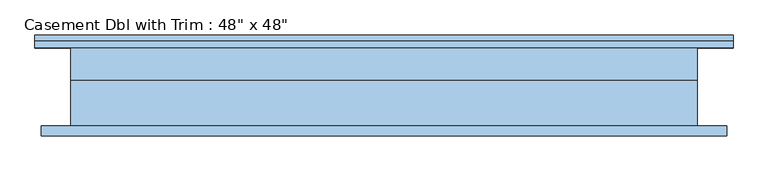
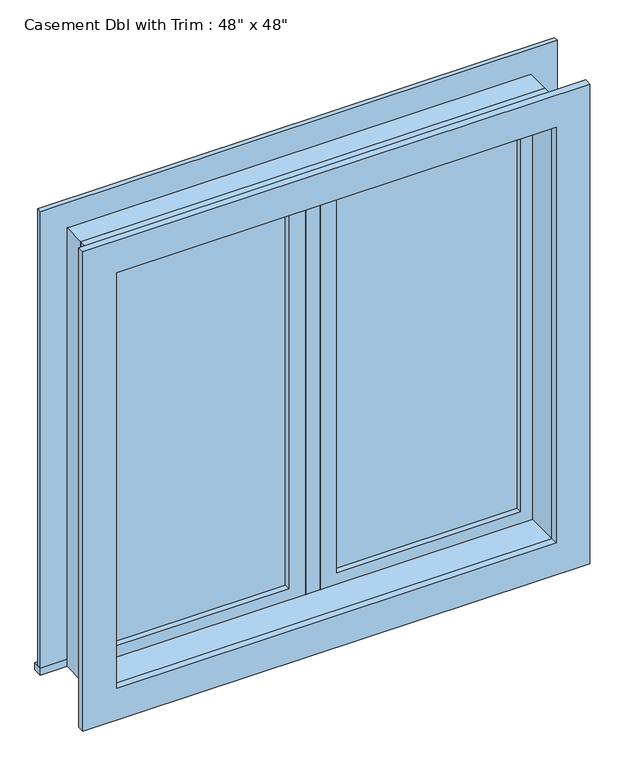
"""IFC4 building model written with IfcOpenShell, lengths in millimetres: window geometry."""

from ifc_helpers import new_model, si_unit, frame, origin, place, context, project, spatial, polyline, outline, extrude, source, transform, mapped, element, save


def window_be30da88(model_context):
    return source(origin(), model_context, "Body", "SweptSolid", [
        extrude(outline(polyline([(63.5, 60.325), (546.1, 60.325), (546.1, 47.625), (63.5, 47.625), (63.5, 60.325)])), frame((0.0, 0.0, 977.9), z_axis=(0.0, 0.0, 1.0), x_axis=(1.0, 0.0, 0.0)), (0.0, 0.0, 1.0), 1092.2),
        extrude(outline(polyline([(2114.55, 19.05), (933.45, 19.05), (933.45, 590.55), (2114.55, 590.55), (2114.55, 19.05)]), holes=[polyline([(2070.1, 63.5), (2070.1, 546.1), (977.9, 546.1), (977.9, 63.5), (2070.1, 63.5)])]), frame((0.0, 31.75, 0.0), z_axis=(0.0, 1.0, 0.0), x_axis=(0.0, 0.0, 1.0)), (0.0, 0.0, 1.0), 44.45),
        extrude(outline(polyline([(19.05, 31.75), (-19.05, 31.75), (-19.05, 95.25), (19.05, 95.25), (19.05, 31.75)])), frame((0.0, 0.0, 933.45), z_axis=(0.0, 0.0, 1.0), x_axis=(1.0, 0.0, 0.0)), (0.0, 0.0, 1.0), 1181.1),
        extrude(outline(polyline([(-679.45, 120.65), (679.45, 120.65), (679.45, 95.25), (-679.45, 95.25), (-679.45, 120.65)])), frame((0.0, 0.0, 914.4), z_axis=(0.0, 0.0, 1.0), x_axis=(1.0, 0.0, 0.0)), (0.0, 0.0, 1.0), 19.05),
        extrude(outline(polyline([(2114.55, -590.55), (2114.55, 590.55), (933.45, 590.55), (933.45, 679.45), (2203.45, 679.45), (2203.45, -679.45), (933.45, -679.45), (933.45, -590.55), (2114.55, -590.55)])), frame((0.0, 95.25, 0.0), z_axis=(0.0, 1.0, 0.0), x_axis=(0.0, 0.0, 1.0)), (0.0, 0.0, 1.0), 12.7),
        extrude(outline(polyline([(2190.75, 666.75), (2190.75, -666.75), (857.25, -666.75), (857.25, 666.75), (2190.75, 666.75)]), holes=[polyline([(2101.85, 577.85), (946.15, 577.85), (946.15, -577.85), (2101.85, -577.85), (2101.85, 577.85)])]), frame((0.0, -76.2, 0.0), z_axis=(0.0, 1.0, 0.0), x_axis=(0.0, 0.0, 1.0)), (0.0, 0.0, 1.0), 19.05),
        extrude(outline(polyline([(-63.5, 47.625), (-546.1, 47.625), (-546.1, 60.325), (-63.5, 60.325), (-63.5, 47.625)])), frame((0.0, 0.0, 977.9), z_axis=(0.0, 0.0, 1.0), x_axis=(1.0, 0.0, 0.0)), (0.0, 0.0, 1.0), 1092.2),
        extrude(outline(polyline([(2114.55, -590.55), (933.45, -590.55), (933.45, -19.05), (2114.55, -19.05), (2114.55, -590.55)]), holes=[polyline([(2070.1, -546.1), (2070.1, -63.5), (977.9, -63.5), (977.9, -546.1), (2070.1, -546.1)])]), frame((0.0, 31.75, 0.0), z_axis=(0.0, 1.0, 0.0), x_axis=(0.0, 0.0, 1.0)), (0.0, 0.0, 1.0), 44.45),
        extrude(outline(polyline([(2133.6, -609.6), (914.4, -609.6), (914.4, 609.6), (2133.6, 609.6), (2133.6, -609.6)]), holes=[polyline([(2101.85, -577.85), (2101.85, 577.85), (946.15, 577.85), (946.15, -577.85), (2101.85, -577.85)])]), frame((0.0, -57.15, 0.0), z_axis=(0.0, 1.0, 0.0), x_axis=(0.0, 0.0, 1.0)), (0.0, 0.0, 1.0), 88.9),
        extrude(outline(polyline([(2133.6, 609.6), (2133.6, -609.6), (914.4, -609.6), (914.4, 609.6), (2133.6, 609.6)]), holes=[polyline([(2114.55, 590.55), (933.45, 590.55), (933.45, -590.55), (2114.55, -590.55), (2114.55, 590.55)])]), frame((0.0, 31.75, 0.0), z_axis=(0.0, 1.0, 0.0), x_axis=(0.0, 0.0, 1.0)), (0.0, 0.0, 1.0), 63.5),
    ])


if __name__ == "__main__":
    model = new_model("IFC4")
    model_context = context("Model", 3, world=origin())
    ifc_project = project(units=[si_unit("LENGTHUNIT", "METRE", prefix="MILLI")], contexts=[model_context])
    site = spatial("IfcSite", under=ifc_project)
    building = spatial("IfcBuilding", under=site)
    placement = place(None, origin())
    window_shape = window_be30da88(model_context)
    element("IfcWindow", 1, ObjectType="Casement Dbl with Trim : 48\" x 48\"", at=placement, inside=building, context=model_context, shape_type="MappedRepresentation", body=[
        mapped(window_shape, transform((0.0, 0.0, 0.0), x_axis=(1.0, 0.0, 0.0), y_axis=(0.0, 1.0, 0.0), z_axis=(0.0, 0.0, 1.0))),
    ])
    save(model, "model.ifc")

# Revit data of these elements
# Type "Casement Dbl with Trim : 48\" x 48\""
#   Type Mark = "10"
#   Construction Type Id = "GSP4R"
#   Assembly Code = "B2020100"
#   Analytic Construction = "1/8 in Pilkington single glazing"
#   Visual Light Transmittance = 0.9
#   Solar Heat Gain Coefficient = 0.78
#   Heat Transfer Coefficient (U) = 0.6496 BTU/(h·ft²·°F)
#   Height = 4' - 0"
#   Default Sill Height = 3' - 0"
#   Trim Projection - Ext. = 0' - 0 1/2"
#   Trim Projection - Int. = 0' - 0 3/4"
#   Trim Width - Exterior = 0' - 3 1/2"
#   Trim Width - Interior = 0' - 3 1/2"
#   Width = 4' - 0"
#   Window Inset = 0' - 0 3/4"
#   Define Thermal Properties by = 1
#   Glass Pane Material = Glass
#   Sash Material = Sash
#   Trim Exterior Material = Trim
#   Trim Interior Material = Trim
#   Wall Closure = (empty or 0)
# Element 1 (IfcWindow, "Casement Dbl with Trim : 48\" x 48\"")
#   Materials on its faces: "Sash", "Trim", "Glass"
# Materials
#   "Glass": class "Glass", colour RGB 0 128 192, transparency 0.75, Description = "Soda Lime Glass", Cost = 0
#   "Sash": class "Wood", colour RGB 224 178 126, transparency 0
#   "Trim": class "Wood", colour RGB 224 178 126, transparency 0
